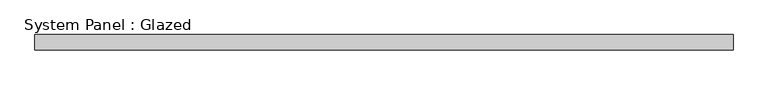
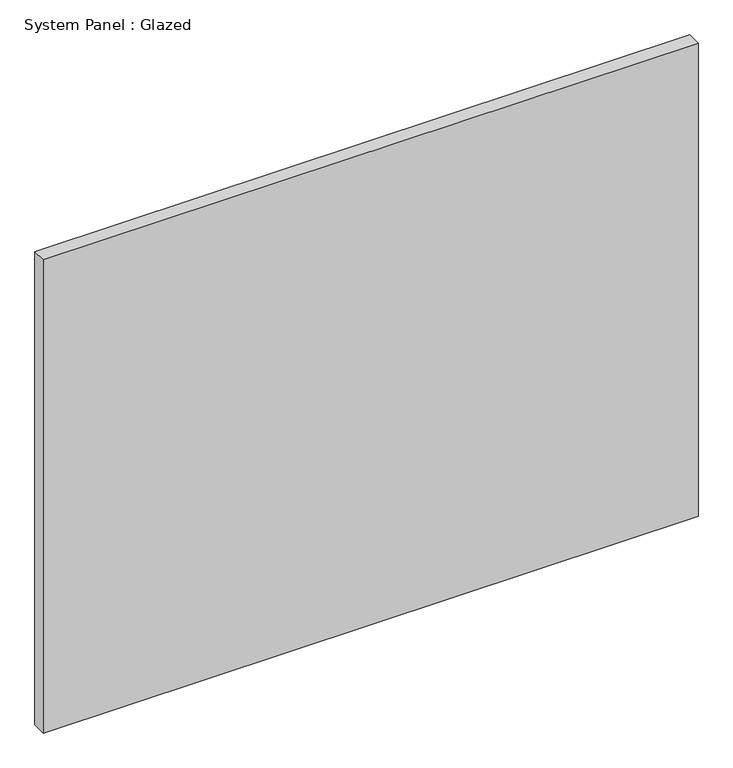
"""IFC4 building model written with IfcOpenShell, lengths in millimetres: plate geometry, System Panel : Glazed."""

from ifc_helpers import new_model, si_unit, origin, origin_with_axes, place, context, project, spatial, polyline, outline, extrude, source, transform, mapped, element, save


def system_panel_glazed_d871acfc(model_context):
    return source(origin(), model_context, "Body", "SweptSolid", [
        extrude(outline(polyline([(587.375, 19.05), (-587.375, 19.05), (-587.375, 44.45), (587.375, 44.45), (587.375, 19.05)])), origin_with_axes(), (0.0, 0.0, 1.0), 897.3037122),
    ])


if __name__ == "__main__":
    model = new_model("IFC4")
    model_context = context("Model", 3, world=origin())
    ifc_project = project(units=[si_unit("LENGTHUNIT", "METRE", prefix="MILLI")], contexts=[model_context])
    site = spatial("IfcSite", under=ifc_project)
    building = spatial("IfcBuilding", under=site)
    placement = place(None, origin())
    system_panel_glazed_shape = system_panel_glazed_d871acfc(model_context)
    element("IfcPlate", 1, ObjectType="System Panel : Glazed", at=placement, inside=building, context=model_context, shape_type="MappedRepresentation", body=[
        mapped(system_panel_glazed_shape, transform((0.0, 0.0, 0.0), x_axis=(1.0, 0.0, 0.0), y_axis=(0.0, 1.0, 0.0), z_axis=(0.0, 0.0, 1.0))),
    ])
    save(model, "model.ifc")

# Revit data of these elements
# Type "System Panel : Glazed"
#   Construction Type Id = "GSP4R"
#   Analytic Construction = "1/8 in Pilkington single glazing"
#   Visual Light Transmittance = 0.9
#   Solar Heat Gain Coefficient = 0.86
#   Heat Transfer Coefficient (U) = 1.18115 BTU/(h·ft²·°F)
#   Define Thermal Properties by = 1
# Element 1 (IfcPlate, "System Panel : Glazed")
#   Materials on its faces: "Glass"
# Materials
#   "Glass": class "Glass", colour RGB 0 128 192, transparency 0.75, Description = "Soda Lime Glass", Cost = 0
